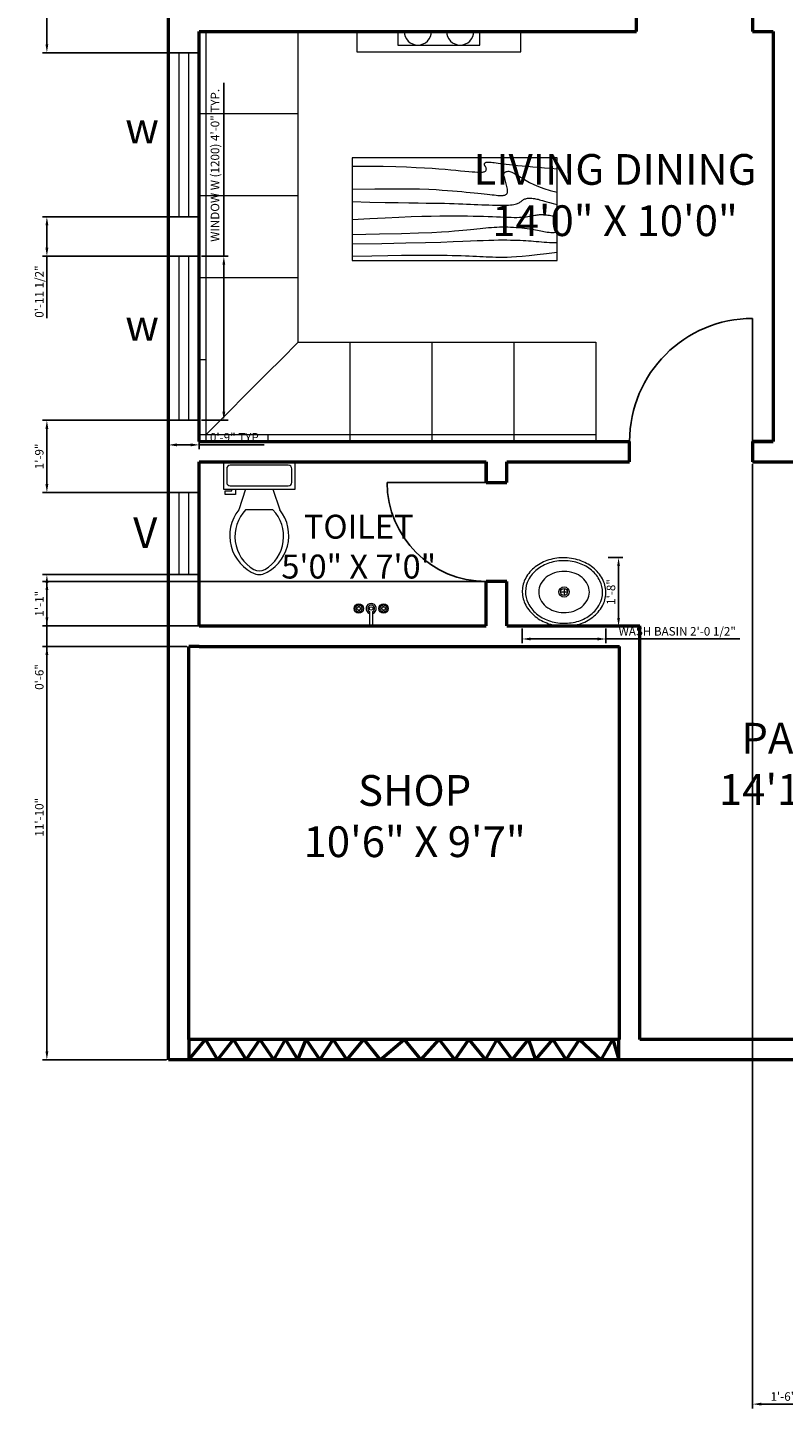
# Model space of a CAD drawing. Units: inches. Extents: x 3688 to 4628, y 1593 to 2337.
# Tile 1 of 7: x 3688 to 3910, y 1593 to 1997. Entities that reach past the tile are written whole.
import ezdxf

# ---------------------------------------------------------------- set-up
doc = ezdxf.new("R2010")
doc.units = ezdxf.units.IN
for name, color, linetype, lineweight in [('A-ANNO-DIMS', 2, 'Continuous', 18), ('A-ANNO-TEXT', 7, 'Continuous', 18), ('A-AREA-IDEN', 7, 'Continuous', 25), ('A-DOOR', 4, 'Continuous', 25), ('A-FLOR-FIXT', 8, 'Continuous', 18), ('A-FURN', 8, 'Continuous', 18), ('A-GLAZ', 4, 'Continuous', 25), ('A-WALL', 7, 'Continuous', 50)]:
    doc.layers.add(name, color=color, linetype=linetype, lineweight=lineweight)
doc.styles.get("Standard").update_dxf_attribs({"font": 'arial.ttf'})
doc.dimstyles.new('ISO-25', dxfattribs={"dimtxt": 2.5, "dimasz": 2.5, "dimexe": 1.25, "dimexo": 0.625, "dimtad": 1, "dimdec": 0, "dimlunit": 3, "dimtxsty": 'Standard', "dimcen": 2.5, "dimadec": 0, "dimazin": 0, "dimtfac": 1, "dimtdec": 0, "dimtmove": 0, "dimatfit": 3, "dimfxl": 1, "dimarcsym": 0})

# ---------------------------------------------------------------- blocks, each defined once
blk = doc.blocks.new('Sink - Oval top')
for p, q in [((-1, 0), (1, 0)), ((0, 1), (0, -1))]:
    blk.add_line(p, q)
for points in [[(-12.23, 0.39, 0.117634), (-11.46, -3.36, 0.104469), (-8.88, -6.8, 0.090016), (-5.08, -9.07, 0.08192), (-0.32, -10.02, 0.08192), (4.49, -9.38, 0.090016), (8.42, -7.36, 0.104469), (11.22, -4.09, 0.117634), (12.23, -0.39, 0.117634), (11.46, 3.36, 0.104469), (8.88, 6.8, 0.090016), (5.08, 9.07, 0.08192), (0.32, 10.02, 0.08192), (-4.49, 9.38, 0.090016), (-8.42, 7.36, 0.104469), (-11.22, 4.09, 0.117634)], [(-11.29, 0.16, 0.118622), (-10.52, -3.25, 0.104678), (-8.07, -6.36, 0.089562), (-4.54, -8.37, 0.081185), (-0.13, -9.15, 0.081185), (4.3, -8.49, 0.089562), (7.89, -6.58, 0.104678), (10.42, -3.55, 0.118622), (11.29, -0.16, 0.118622), (10.52, 3.25, 0.104678), (8.07, 6.36, 0.089562), (4.54, 8.37, 0.081185), (0.13, 9.15, 0.081185), (-4.3, 8.49, 0.089562), (-7.89, 6.58, 0.104678), (-10.42, 3.55, 0.118622)], [(-7.42, 0.08, 0.118283), (-6.91, -2.17, 0.104607), (-5.29, -4.21, 0.089718), (-2.97, -5.53, 0.081436), (-0.07, -6.04, 0.081436), (2.84, -5.59, 0.089718), (5.2, -4.33, 0.104607), (6.86, -2.32, 0.118283), (7.42, -0.08, 0.118283), (6.91, 2.17, 0.104607), (5.29, 4.21, 0.089718), (2.97, 5.53, 0.081436), (0.07, 6.04, 0.081436), (-2.84, 5.59, 0.089718), (-5.2, 4.33, 0.104607), (-6.86, 2.32, 0.118283)]]:
    blk.add_lwpolyline(points, format="xyb", close=True)
for radius in [1.5, 1]:
    blk.add_circle((0, 0), radius)
blk = doc.blocks.new('Toilet - top')
for p, q in [((9.5, -6), (9.5, -2)), ((-8, -8.5), (-8, -8)), ((-7, -8), (-7, -9.5)), ((-4, -8), (-6, -14)), ((4, -8), (6, -14)), ((-10, -8.5), (-8, -8.5)), ((-10, -9.5), (-10, -8.5)), ((-7, -9.5), (-10, -9.5)), ((4, -14), (-4, -14))]:
    blk.add_line(p, q)
blk.add_lwpolyline([(10.5, -8), (10.5, 0), (-10.5, 0), (-10.5, -8)], close=True)
for points in [[(-9.5, -2), (-9.5, -6)], [(8.5, -1), (-8.5, -1)], [(-8.5, -7), (8.5, -7)]]:
    blk.add_lwpolyline(points)
for centre, radius, start, end in [((-8.62, -1.88), 0.884, 81.8699, 188.1301), ((8.62, -1.88), 0.884, 351.8699, 98.1301), ((-8.62, -6.12), 0.884, 171.8699, 278.1301), ((8.62, -6.12), 0.884, 261.8699, 8.1301), ((3.52, -21.58), 12.17, 141.4691, 247.9714), ((4.2, -21.82), 11.33, 136.3677, 238.9468), ((-3.52, -21.58), 12.17, 292.0284, 38.5307), ((-4.2, -21.82), 11.33, 301.053, 43.6321), ((0, -27.88), 4, 245.7318, 294.2682), ((0, -29), 4, 254.8605, 285.1395)]:
    blk.add_arc(centre, radius, start, end)
blk = doc.blocks.new('Table - Rectangular Woodgrain 60 x 30 in.')
for p, q in [((0, 0), (0, -30)), ((60, 0), (0, 0)), ((60, -30), (60, 0)), ((0, -30), (60, -30))]:
    blk.add_line(p, q)
for points in [[(0, -2.4), (4.8155, -2.418), (9.0302, -2.4688), (12.709, -2.5477), (15.9167, -2.65), (18.7181, -2.7711), (21.1781, -2.9063), (23.3616, -3.0508), (25.3333, -3.2), (27.1477, -3.3495), (28.8172, -3.4958), (30.3437, -3.636), (31.7291, -3.7667), (32.9756, -3.8849), (34.0849, -3.9875), (35.059, -4.0714), (35.9, -4.1334), (36.6114, -4.1711), (37.2041, -4.1854), (37.6906, -4.1779), (38.0833, -4.15), (38.3948, -4.1034), (38.6375, -4.0396), (38.8239, -3.9602), (38.9666, -3.8667), (39.0764, -3.7608), (39.1573, -3.6448), (39.2116, -3.521), (39.2416, -3.3917), (39.2498, -3.2593), (39.2385, -3.1261), (39.21, -2.9944), (39.1666, -2.8667), (39.111, -2.7447), (39.0468, -2.6281), (38.978, -2.5163), (38.9083, -2.4083), (38.8418, -2.3035), (38.7823, -2.201), (38.7337, -2.1001), (38.7, -2), (38.6844, -1.9003), (38.6875, -1.8021), (38.7094, -1.707), (38.75, -1.6167), (38.8094, -1.5326), (38.8875, -1.4563), (38.9844, -1.3893), (39.1, -1.3333), (39.2351, -1.2896), (39.3937, -1.2583), (39.5804, -1.2396), (39.8, -1.2333), (40.057, -1.2396), (40.3562, -1.2583), (40.7023, -1.2896), (41.1, -1.3333), (41.5547, -1.3895), (42.0755, -1.4573), (42.6721, -1.5361), (43.3542, -1.625), (44.1316, -1.7233), (45.014, -1.8302), (46.0114, -1.9449), (47.1333, -2.0667), (48.3862, -2.1947), (49.7625, -2.3281), (51.2513, -2.4663), (52.8416, -2.6083), (54.5226, -2.7535), (56.2833, -2.9011), (58.1127, -3.0501), (60, -3.2)], [(0, -9.2), (6.5759, -9.0858), (11.9385, -9.0365), (16.2527, -9.0418), (19.6833, -9.0917), (22.3952, -9.1759), (24.5531, -9.2844), (26.322, -9.4069), (27.8666, -9.5333), (29.3241, -9.6553), (30.7203, -9.7719), (32.0532, -9.8837), (33.3208, -9.9917), (34.5213, -10.0965), (35.6526, -10.199), (36.7128, -10.2999), (37.7, -10.4), (38.6129, -10.4996), (39.4531, -10.5969), (40.223, -10.6895), (40.925, -10.775), (41.5613, -10.8512), (42.1344, -10.9156), (42.6465, -10.966), (43.1, -11), (43.4976, -11.0158), (43.8437, -11.0136), (44.143, -10.9942), (44.4, -10.9583), (44.6195, -10.9069), (44.8062, -10.8406), (44.9648, -10.7603), (45.1, -10.6667), (45.2155, -10.5598), (45.3114, -10.4365), (45.3871, -10.2929), (45.4416, -10.125), (45.4743, -9.929), (45.4844, -9.7011), (45.4709, -9.4371), (45.4333, -9.1333), (45.3716, -8.7883), (45.2896, -8.4104), (45.1919, -8.0107), (45.0833, -7.6), (44.9685, -7.1893), (44.8521, -6.7896), (44.7388, -6.4117), (44.6333, -6.0667), (44.54, -5.7628), (44.4614, -5.4979), (44.4001, -5.2675), (44.3583, -5.0667), (44.3384, -4.8909), (44.3427, -4.7354), (44.3736, -4.5956), (44.4333, -4.4667), (44.5236, -4.3453), (44.6427, -4.2333), (44.7884, -4.1339), (44.9583, -4.05), (45.1501, -3.9849), (45.3614, -3.9417), (45.59, -3.9234), (45.8333, -3.9333), (46.0915, -3.9749), (46.3734, -4.0531), (46.6906, -4.1736), (47.0542, -4.3417), (47.4756, -4.5629), (47.9661, -4.8427), (48.5372, -5.1866), (49.2, -5.6), (49.9676, -6.0844), (50.8594, -6.625), (51.8965, -7.2031), (53.1, -7.8), (54.491, -8.3969), (56.0906, -8.975), (57.9199, -9.5156), (60, -10)], [(0, -12.8), (5.1847, -12.9322), (9.6213, -13.0323), (13.3963, -13.1059), (16.5958, -13.1583), (19.3063, -13.1952), (21.614, -13.2219), (23.6054, -13.2439), (25.3666, -13.2667), (26.9728, -13.2947), (28.4531, -13.3281), (29.8256, -13.3663), (31.1083, -13.4083), (32.3191, -13.4535), (33.476, -13.501), (34.597, -13.5501), (35.7, -13.6), (36.7984, -13.6497), (37.8875, -13.6979), (38.9578, -13.743), (40, -13.7833), (41.0047, -13.8174), (41.9625, -13.8438), (42.864, -13.8607), (43.7, -13.8667), (44.4631, -13.8604), (45.1552, -13.8417), (45.7801, -13.8104), (46.3416, -13.7667), (46.8439, -13.7104), (47.2906, -13.6417), (47.6858, -13.5604), (48.0333, -13.4667), (48.3375, -13.3608), (48.6042, -13.2448), (48.8396, -13.121), (49.05, -12.9917), (49.2417, -12.8593), (49.4208, -12.7261), (49.5937, -12.5944), (49.7667, -12.4667), (49.9452, -12.3451), (50.1323, -12.2313), (50.3303, -12.1268), (50.5416, -12.0333), (50.7686, -11.9524), (51.0135, -11.8854), (51.2788, -11.8341), (51.5666, -11.8), (51.8785, -11.7843), (52.2116, -11.7865), (52.562, -11.8059), (52.926, -11.8417), (53.2998, -11.8931), (53.6795, -11.9594), (54.0614, -12.0397), (54.4416, -12.1333), (54.8223, -12.2401), (55.2293, -12.3625), (55.6942, -12.5037), (56.2489, -12.6667), (56.9251, -12.8547), (57.7545, -13.0708), (58.7689, -13.3182), (60, -13.6)], [(0, -18), (5.124, -17.7273), (9.6609, -17.5057), (13.6705, -17.3303), (17.2125, -17.1958), (20.3467, -17.0973), (23.1328, -17.0297), (25.6307, -16.9878), (27.9, -16.9667), (29.9928, -16.9617), (31.9302, -16.9703), (33.7254, -16.9907), (35.3917, -17.0208), (36.9423, -17.0588), (38.3906, -17.1026), (39.7499, -17.1503), (41.0333, -17.2), (42.2519, -17.2496), (43.4073, -17.2969), (44.4986, -17.3395), (45.525, -17.375), (46.4858, -17.4012), (47.3802, -17.4156), (48.2074, -17.416), (48.9667, -17.4), (49.6583, -17.3662), (50.2872, -17.3167), (50.8595, -17.2547), (51.3812, -17.1833), (51.8584, -17.1057), (52.2971, -17.025), (52.7034, -16.9443), (53.0833, -16.8667), (53.443, -16.7951), (53.789, -16.7313), (54.128, -16.6768), (54.4666, -16.6334), (54.8115, -16.6024), (55.1693, -16.5854), (55.5465, -16.5841), (55.95, -16.6), (56.3828, -16.6337), (56.8346, -16.6823), (57.2915, -16.7418), (57.7396, -16.8084), (58.165, -16.878), (58.5539, -16.9469), (58.8924, -17.0111), (59.1666, -17.0667), (59.3679, -17.1107), (59.5078, -17.1438), (59.6032, -17.1675), (59.6708, -17.1833), (59.7275, -17.193), (59.7901, -17.1979), (59.8753, -17.1998), (60, -17.2)], [(0, -22.4), (8.0098, -22.2501), (14.4094, -22.1011), (19.4168, -21.9535), (23.25, -21.8083), (26.1269, -21.6663), (28.2656, -21.5281), (29.884, -21.3947), (31.2, -21.2667), (32.3967, -21.1448), (33.5172, -21.0292), (34.5697, -20.9198), (35.5625, -20.8167), (36.5037, -20.7198), (37.4015, -20.6292), (38.2642, -20.5448), (39.1, -20.4667), (39.9164, -20.3951), (40.7187, -20.3313), (41.5117, -20.2768), (42.3, -20.2333), (43.0883, -20.2024), (43.8812, -20.1854), (44.6836, -20.1841), (45.5, -20.2), (46.3328, -20.234), (47.1747, -20.2844), (48.0163, -20.3488), (48.8479, -20.425), (49.66, -20.5106), (50.4429, -20.6031), (51.1872, -20.7004), (51.8833, -20.8), (52.5246, -20.8999), (53.1166, -20.9995), (53.6681, -21.0983), (54.1875, -21.1958), (54.6834, -21.2919), (55.1646, -21.3859), (55.6394, -21.4777), (56.1167, -21.5667), (56.6028, -21.6515), (57.0961, -21.7266), (57.5929, -21.7852), (58.0896, -21.8208), (58.5823, -21.8268), (59.0674, -21.7964), (59.5412, -21.723), (60, -21.6)], [(0, -25.2), (8.6355, -25.0504), (15.7026, -24.9031), (21.4049, -24.7606), (25.9458, -24.625), (29.529, -24.4988), (32.3578, -24.3844), (34.6359, -24.284), (36.5667, -24.2), (38.3213, -24.1341), (39.9417, -24.0854), (41.437, -24.0523), (42.8167, -24.0333), (44.0901, -24.0268), (45.2667, -24.0313), (46.3557, -24.0451), (47.3667, -24.0667), (48.309, -24.0947), (49.1928, -24.1287), (50.0284, -24.168), (50.826, -24.2125), (51.5959, -24.2617), (52.3483, -24.3151), (53.0935, -24.3725), (53.8417, -24.4334), (54.6009, -24.497), (55.3699, -24.561), (56.1454, -24.6226), (56.9239, -24.6792), (57.7021, -24.7279), (58.4764, -24.7662), (59.2435, -24.7911), (60, -24.8)], [(0, -28.8), (5.6867, -28.6681), (10.45, -28.5698), (14.407, -28.5012), (17.675, -28.4584), (20.3711, -28.4374), (22.6125, -28.4344), (24.5164, -28.4455), (26.2, -28.4667), (27.762, -28.4947), (29.2276, -28.5281), (30.6033, -28.5663), (31.8958, -28.6084), (33.1118, -28.6535), (34.2578, -28.7011), (35.3405, -28.7501), (36.3666, -28.8), (37.3443, -28.8497), (38.288, -28.8974), (39.2137, -28.9412), (40.1375, -28.9792), (41.0753, -29.0093), (42.0432, -29.0297), (43.0572, -29.0384), (44.1333, -29.0333), (45.2936, -29.0114), (46.5843, -28.9641), (48.0579, -28.8816), (49.7666, -28.7542), (51.7629, -28.5721), (54.0989, -28.3255), (56.8272, -28.0048), (60, -27.6)]]:
    blk.add_lwpolyline(points)
blk = doc.blocks.new('Faucet - Bathroom top')
for p, q in [((-4.107, 0.125), (-4.375, 0.125)), ((-3.75, 0.4788), (-3.75, 0.75)), ((-3.5, 0.482), (-3.5, 0.75)), ((-3.1461, 0.125), (-2.875, 0.125)), ((3.143, 0.125), (2.875, 0.125)), ((3.5, 0.4788), (3.5, 0.75)), ((3.75, 0.482), (3.75, 0.75)), ((4.1039, 0.125), (4.375, 0.125)), ((-4.1039, -0.125), (-4.375, -0.125)), ((-3.75, -0.4821), (-3.75, -0.75)), ((-3.5, -0.4789), (-3.5, -0.75)), ((-3.143, -0.125), (-2.875, -0.125)), ((-0.5, -0.8639), (-0.5, -4.5)), ((0.5, -4.5), (0.5, -0.8631)), ((3.1461, -0.125), (2.875, -0.125)), ((3.5, -0.4821), (3.5, -0.75)), ((3.75, -0.4789), (3.75, -0.75)), ((4.107, -0.125), (4.375, -0.125))]:
    blk.add_line(p, q)
for centre, radius in [((-3.625, 0), 1.375), ((-4.625, 0), 0.2795), ((-3.625, 0), 0.5), ((-3.625, 1), 0.2795), ((-2.625, 0), 0.2795), ((0, 0), 0.5), ((3.625, 0), 1.375), ((2.625, 0), 0.2795), ((3.625, 0), 0.5), ((3.625, 1), 0.2795), ((4.625, 0), 0.2795), ((-3.625, -1), 0.2795), ((3.625, -1), 0.2795)]:
    blk.add_circle(centre, radius)
for centre, radius, start, end in [((-3.625, 0), 1, 105.2407, 164.2093), ((-3.625, 0), 1, 16.44125, 74.07887), ((0, 0), 1.5, 289.6514, 250.3603), ((0, 0), 1, 300.3431, 239.7554), ((3.625, 0), 1, 106.12, 164.0884), ((3.625, 0), 1, 16.23422, 73.90469), ((-3.625, 0), 1, 196.2342, 253.9047), ((-3.625, 0), 1, 286.12, 344.0884), ((3.625, 0), 1, 196.4413, 254.0789), ((3.625, 0), 1, 285.2407, 344.2093), ((0, -4.5), 0.5, 180, 0)]:
    blk.add_arc(centre, radius, start, end)
blk = doc.blocks.new('DOOR-900')
blk.add_line((0, 0), (0, 36))
blk.add_arc((0, 0), 36, 0, 90)
blk = doc.blocks.new('DOOR-750')
blk.add_line((29, 0), (29, 29))
blk.add_arc((29, 0), 29, 90, 180)
blk = doc.blocks.new('WIN-1200')
for p, q in [((0, 48), (0, 0)), ((9, 48), (0, 48)), ((9, 0), (9, 48)), ((0, 0), (9, 0))]:
    blk.add_line(p, q)
blk = doc.blocks.new('WIN-600')
for p, q in [((24, 9), (0, 9)), ((0, 9), (0, 0)), ((24, 0), (24, 9)), ((0, 0), (24, 0))]:
    blk.add_line(p, q)
blk = doc.blocks.new('*D23')
at = {"layer": 'A-ANNO-DIMS', "color": 0, "lineweight": -2, "transparency": 16777216}
for p, q in [((3745.82, 1930.49), (3745.82, 1981.21)), ((3739.25, 1930.49), (3747.07, 1930.49)), ((3745.82, 1884.99), (3745.82, 1927.99)), ((3739.25, 1882.49), (3747.07, 1882.49))]:
    blk.add_line(p, q, dxfattribs=at)
at = {"layer": 'A-ANNO-DIMS', "color": 0, "transparency": 16777216}
for points in [[(3745.41, 1927.99), (3746.24, 1927.99), (3745.82, 1930.49)], [(3745.41, 1884.99), (3746.24, 1884.99), (3745.82, 1882.49)]]:
    blk.add_solid(points, dxfattribs=at)
at = {"layer": 'Defpoints', "color": 0, "transparency": 16777216}
for p in [(3738.62, 1930.49), (3745.82, 1930.49), (3738.62, 1882.49)]:
    blk.add_point(p, dxfattribs=at)
at = {"layer": 'A-ANNO-DIMS', "color": 0, "transparency": 16777216, "insert": (3743.56, 1957.1), "char_height": 2.5, "attachment_point": 5, "rotation": 90}
blk.add_mtext('WINDOW W (1200) 4\'-0" TYP.', dxfattribs=at)
blk = doc.blocks.new('*D24')
at = {"layer": 'A-ANNO-DIMS', "color": 0, "lineweight": -2, "transparency": 16777216}
for p, q in [((3729.62, 1881.87), (3729.62, 1874.04)), ((3738.62, 1881.87), (3738.62, 1874.04)), ((3732.12, 1875.29), (3736.12, 1875.29)), ((3738.62, 1875.29), (3757.61, 1875.29))]:
    blk.add_line(p, q, dxfattribs=at)
at = {"layer": 'A-ANNO-DIMS', "color": 0, "transparency": 16777216}
for points in [[(3732.12, 1875.71), (3732.12, 1874.87), (3729.62, 1875.29)], [(3736.12, 1875.71), (3736.12, 1874.87), (3738.62, 1875.29)]]:
    blk.add_solid(points, dxfattribs=at)
at = {"layer": 'Defpoints', "color": 0, "transparency": 16777216}
for p in [(3729.62, 1882.49), (3738.62, 1882.49), (3738.62, 1875.29)]:
    blk.add_point(p, dxfattribs=at)
at = {"layer": 'A-ANNO-DIMS', "color": 0, "transparency": 16777216, "insert": (3749.37, 1877.19), "char_height": 2.5, "attachment_point": 5}
blk.add_mtext('0\'-9" TYP.', dxfattribs=at)
blk = doc.blocks.new('*D47')
at = {"layer": 'A-ANNO-DIMS', "color": 0, "lineweight": -2, "transparency": 16777216}
for p, q in [((3833.14, 1821.55), (3833.14, 1817.24)), ((3835.64, 1818.49), (3855.19, 1818.49)), ((3857.69, 1821.55), (3857.69, 1817.24)), ((3857.69, 1818.49), (3896.91, 1818.49))]:
    blk.add_line(p, q, dxfattribs=at)
at = {"layer": 'A-ANNO-DIMS', "color": 0, "transparency": 16777216}
for points in [[(3835.64, 1818.91), (3835.64, 1818.07), (3833.14, 1818.49)], [(3855.19, 1818.91), (3855.19, 1818.07), (3857.69, 1818.49)]]:
    blk.add_solid(points, dxfattribs=at)
at = {"layer": 'Defpoints', "color": 0, "transparency": 16777216}
for p in [(3833.14, 1822.17), (3857.69, 1822.17), (3857.69, 1818.49)]:
    blk.add_point(p, dxfattribs=at)
at = {"layer": 'A-ANNO-DIMS', "color": 0, "transparency": 16777216, "insert": (3878.55, 1820.41), "char_height": 2.5, "attachment_point": 5}
blk.add_mtext('WASH BASIN 2\'-0 1/2"', dxfattribs=at)
blk = doc.blocks.new('*D48')
at = {"layer": 'A-ANNO-DIMS', "color": 0, "lineweight": -2, "transparency": 16777216}
for p, q in [((3858.31, 1842.31), (3862.62, 1842.31)), ((3861.37, 1824.67), (3861.37, 1839.81)), ((3858.31, 1822.17), (3862.62, 1822.17))]:
    blk.add_line(p, q, dxfattribs=at)
at = {"layer": 'A-ANNO-DIMS', "color": 0, "transparency": 16777216}
for points in [[(3860.96, 1839.81), (3861.79, 1839.81), (3861.37, 1842.31)], [(3860.96, 1824.67), (3861.79, 1824.67), (3861.37, 1822.17)]]:
    blk.add_solid(points, dxfattribs=at)
at = {"layer": 'Defpoints', "color": 0, "transparency": 16777216}
for p in [(3857.69, 1842.31), (3861.37, 1842.31), (3857.69, 1822.17)]:
    blk.add_point(p, dxfattribs=at)
at = {"layer": 'A-ANNO-DIMS', "color": 0, "transparency": 16777216, "insert": (3859.47, 1832.24), "char_height": 2.5, "attachment_point": 5, "rotation": 90}
blk.add_mtext('1\'-8"', dxfattribs=at)
blk = doc.blocks.new('*D53')
at = {"layer": 'A-ANNO-DIMS', "color": 0, "lineweight": -2, "transparency": 16777216}
for p, q in [((3729, 2029.26), (3692.77, 2029.26)), ((3694.02, 2026.76), (3694.02, 1992.54)), ((3729, 1990.04), (3692.77, 1990.04))]:
    blk.add_line(p, q, dxfattribs=at)
at = {"layer": 'A-ANNO-DIMS', "color": 0, "transparency": 16777216}
for points in [[(3693.61, 2026.76), (3694.44, 2026.76), (3694.02, 2029.26)], [(3693.61, 1992.54), (3694.44, 1992.54), (3694.02, 1990.04)]]:
    blk.add_solid(points, dxfattribs=at)
at = {"layer": 'Defpoints', "color": 0, "transparency": 16777216}
for p in [(3729.62, 2029.26), (3694.02, 1990.04), (3729.62, 1990.04)]:
    blk.add_point(p, dxfattribs=at)
at = {"layer": 'A-ANNO-DIMS', "color": 0, "transparency": 16777216, "insert": (3692.12, 2009.65), "char_height": 2.5, "attachment_point": 5, "rotation": 90}
blk.add_mtext('3\'-3"', dxfattribs=at)
blk = doc.blocks.new('*D54')
at = {"layer": 'A-ANNO-DIMS', "color": 0, "lineweight": -2, "transparency": 16777216}
for p, q in [((3729, 1942.04), (3692.77, 1942.04)), ((3694.02, 1939.54), (3694.02, 1932.99)), ((3729, 1930.49), (3692.77, 1930.49)), ((3694.02, 1930.49), (3694.02, 1912.33))]:
    blk.add_line(p, q, dxfattribs=at)
at = {"layer": 'A-ANNO-DIMS', "color": 0, "transparency": 16777216}
for points in [[(3693.61, 1939.54), (3694.44, 1939.54), (3694.02, 1942.04)], [(3693.61, 1932.99), (3694.44, 1932.99), (3694.02, 1930.49)]]:
    blk.add_solid(points, dxfattribs=at)
at = {"layer": 'Defpoints', "color": 0, "transparency": 16777216}
for p in [(3729.62, 1942.04), (3694.02, 1930.49), (3729.62, 1930.49)]:
    blk.add_point(p, dxfattribs=at)
at = {"layer": 'A-ANNO-DIMS', "color": 0, "transparency": 16777216, "insert": (3692.11, 1920.16), "char_height": 2.5, "attachment_point": 5, "rotation": 90}
blk.add_mtext('0\'-11 1/2"', dxfattribs=at)
blk = doc.blocks.new('*D55')
at = {"layer": 'A-ANNO-DIMS', "color": 0, "lineweight": -2, "transparency": 16777216}
for p, q in [((3729, 1882.49), (3692.77, 1882.49)), ((3694.02, 1879.99), (3694.02, 1863.83)), ((3729, 1861.33), (3692.77, 1861.33))]:
    blk.add_line(p, q, dxfattribs=at)
at = {"layer": 'A-ANNO-DIMS', "color": 0, "transparency": 16777216}
for points in [[(3693.61, 1879.99), (3694.44, 1879.99), (3694.02, 1882.49)], [(3693.61, 1863.83), (3694.44, 1863.83), (3694.02, 1861.33)]]:
    blk.add_solid(points, dxfattribs=at)
at = {"layer": 'Defpoints', "color": 0, "transparency": 16777216}
for p in [(3729.62, 1882.49), (3694.02, 1861.33), (3729.62, 1861.33)]:
    blk.add_point(p, dxfattribs=at)
at = {"layer": 'A-ANNO-DIMS', "color": 0, "transparency": 16777216, "insert": (3692.12, 1871.91), "char_height": 2.5, "attachment_point": 5, "rotation": 90}
blk.add_mtext('1\'-9"', dxfattribs=at)
blk = doc.blocks.new('*D56')
at = {"layer": 'A-ANNO-DIMS', "color": 0, "lineweight": -2, "transparency": 16777216}
for p, q in [((3729, 1837.33), (3692.77, 1837.33)), ((3694.02, 1834.83), (3694.02, 1697.82)), ((3729, 1695.32), (3692.77, 1695.32))]:
    blk.add_line(p, q, dxfattribs=at)
at = {"layer": 'A-ANNO-DIMS', "color": 0, "transparency": 16777216}
for points in [[(3693.61, 1834.83), (3694.44, 1834.83), (3694.02, 1837.33)], [(3693.61, 1697.82), (3694.44, 1697.82), (3694.02, 1695.32)]]:
    blk.add_solid(points, dxfattribs=at)
at = {"layer": 'Defpoints', "color": 0, "transparency": 16777216}
for p in [(3729.62, 1837.33), (3694.02, 1695.32), (3729.62, 1695.32)]:
    blk.add_point(p, dxfattribs=at)
at = {"layer": 'A-ANNO-DIMS', "color": 0, "transparency": 16777216, "insert": (3692.12, 1766.32), "char_height": 2.5, "attachment_point": 5, "rotation": 90}
blk.add_mtext('11\'-10"', dxfattribs=at)
blk = doc.blocks.new('*D72')
at = {"layer": 'A-ANNO-DIMS', "color": 0, "lineweight": -2, "transparency": 16777216}
for p, q in [((3900.62, 1869.69), (3900.62, 1593.32)), ((3918.62, 1869.69), (3918.62, 1593.32)), ((3903.12, 1594.57), (3916.12, 1594.57))]:
    blk.add_line(p, q, dxfattribs=at)
at = {"layer": 'A-ANNO-DIMS', "color": 0, "transparency": 16777216}
for points in [[(3903.12, 1594.98), (3903.12, 1594.15), (3900.62, 1594.57)], [(3916.12, 1594.98), (3916.12, 1594.15), (3918.62, 1594.57)]]:
    blk.add_solid(points, dxfattribs=at)
at = {"layer": 'Defpoints', "color": 0, "transparency": 16777216}
for p in [(3900.62, 1870.32), (3918.62, 1870.32), (3918.62, 1594.57)]:
    blk.add_point(p, dxfattribs=at)
at = {"layer": 'A-ANNO-DIMS', "color": 0, "transparency": 16777216, "insert": (3909.62, 1596.47), "char_height": 2.5, "attachment_point": 5}
blk.add_mtext('1\'-6"', dxfattribs=at)
blk = doc.blocks.new('*D73')
at = {"layer": 'A-ANNO-DIMS', "color": 0, "lineweight": -2, "transparency": 16777216}
for p, q in [((3694.02, 1824.82), (3694.02, 1827.32)), ((3738, 1822.32), (3692.77, 1822.32)), ((3694.02, 1822.32), (3694.02, 1816.32)), ((3735, 1816.32), (3692.77, 1816.32)), ((3694.02, 1813.82), (3694.02, 1803.42))]:
    blk.add_line(p, q, dxfattribs=at)
at = {"layer": 'A-ANNO-DIMS', "color": 0, "transparency": 16777216}
for points in [[(3693.61, 1824.82), (3694.44, 1824.82), (3694.02, 1822.32)], [(3693.61, 1813.82), (3694.44, 1813.82), (3694.02, 1816.32)]]:
    blk.add_solid(points, dxfattribs=at)
at = {"layer": 'Defpoints', "color": 0, "transparency": 16777216}
for p in [(3738.62, 1822.32), (3694.02, 1816.32), (3735.62, 1816.32)]:
    blk.add_point(p, dxfattribs=at)
at = {"layer": 'A-ANNO-DIMS', "color": 0, "transparency": 16777216, "insert": (3692.12, 1807.37), "char_height": 2.5, "attachment_point": 5, "rotation": 90}
blk.add_mtext('0\'-6"', dxfattribs=at)
blk = doc.blocks.new('*D74')
at = {"layer": 'A-ANNO-DIMS', "color": 0, "lineweight": -2, "transparency": 16777216}
for p, q in [((3822, 1835.32), (3692.77, 1835.32)), ((3694.02, 1832.82), (3694.02, 1824.82)), ((3822, 1822.32), (3692.77, 1822.32))]:
    blk.add_line(p, q, dxfattribs=at)
at = {"layer": 'A-ANNO-DIMS', "color": 0, "transparency": 16777216}
for points in [[(3693.61, 1832.82), (3694.44, 1832.82), (3694.02, 1835.32)], [(3693.61, 1824.82), (3694.44, 1824.82), (3694.02, 1822.32)]]:
    blk.add_solid(points, dxfattribs=at)
at = {"layer": 'Defpoints', "color": 0, "transparency": 16777216}
for p in [(3822.62, 1835.32), (3694.02, 1822.32), (3822.62, 1822.32)]:
    blk.add_point(p, dxfattribs=at)
at = {"layer": 'A-ANNO-DIMS', "color": 0, "transparency": 16777216, "insert": (3692.14, 1828.82), "char_height": 2.5, "attachment_point": 5, "rotation": 90}
blk.add_mtext('1\'-1"', dxfattribs=at)

msp = doc.modelspace()

# ---------------------------------------------------------------- linework, layer by layer
at = {"layer": 'A-FURN'}
for p, q in [((3740.62, 1876.32), (3740.62, 1996.32)), ((3767.62, 1905.32), (3767.62, 1996.32)), ((3784.77, 1996.32), (3784.77, 1993.32)), ((3784.77, 1996.32), (3796.77, 1996.32)), ((3796.77, 1996.32), (3796.77, 1992.32)), ((3820.77, 1992.32), (3820.77, 1996.32)), ((3832.77, 1990.32), (3832.77, 1996.32)), ((3784.77, 1993.32), (3784.77, 1990.32)), ((3796.77, 1992.32), (3820.77, 1992.32)), ((3732.62, 1990.04), (3732.62, 1942.04)), ((3735.62, 1942.04), (3735.62, 1990.04)), ((3784.77, 1990.32), (3832.77, 1990.32)), ((3738.62, 1972.32), (3767.62, 1972.32)), ((3738.62, 1948.32), (3767.62, 1948.32)), ((3732.62, 1930.49), (3732.62, 1882.49)), ((3735.62, 1882.49), (3735.62, 1930.49)), ((3738.62, 1924.32), (3767.62, 1924.32)), ((3767.62, 1905.32), (3762.62, 1900.32)), ((3767.62, 1905.32), (3854.73, 1905.32)), ((3782.73, 1905.32), (3782.73, 1876.32)), ((3806.73, 1905.32), (3806.73, 1876.32)), ((3830.73, 1905.32), (3830.73, 1876.32)), ((3854.73, 1905.32), (3854.73, 1876.32)), ((3738.62, 1900.32), (3740.62, 1900.32)), ((3758.73, 1896.43), (3762.62, 1900.32)), ((3758.73, 1896.43), (3740.62, 1878.32)), ((3738.62, 1878.32), (3854.73, 1878.32)), ((3758.73, 1878.32), (3758.73, 1876.32)), ((3732.62, 1861.33), (3732.62, 1837.33)), ((3735.62, 1837.33), (3735.62, 1861.33))]:
    msp.add_line(p, q, dxfattribs=at)
for centre in [(3802.62, 1996.32), (3815.02, 1996.32)]:
    msp.add_arc(centre, 4, 180, 0, dxfattribs=at)
at = {"layer": 'A-WALL'}
for p, q in [((3729.62, 1695.32), (3729.62, 2295.32)), ((3866.62, 1996.32), (3866.62, 2002.32)), ((3900.62, 2002.32), (3900.62, 1996.32)), ((3738.62, 1996.32), (3866.62, 1996.32)), ((3738.62, 1876.32), (3738.62, 1996.32)), ((3900.62, 1996.32), (3906.62, 1996.32)), ((3906.62, 1996.32), (3906.62, 1876.32)), ((3738.62, 1876.32), (3864.62, 1876.32)), ((3864.62, 1870.32), (3864.62, 1876.32)), ((3906.62, 1876.32), (3900.62, 1876.32)), ((3900.62, 1876.32), (3900.62, 1870.32)), ((3900.62, 1876.32), (3906.62, 1876.32)), ((3738.62, 1870.32), (3798.62, 1870.32)), ((3738.62, 1822.32), (3738.62, 1870.32)), ((3798.62, 1870.32), (3804.62, 1870.32)), ((3804.62, 1870.32), (3822.62, 1870.32)), ((3822.62, 1870.32), (3822.62, 1864.32)), ((3822.62, 1864.32), (3822.62, 1870.32)), ((3828.62, 1870.32), (3864.62, 1870.32)), ((3828.62, 1864.32), (3828.62, 1870.32)), ((3900.62, 1870.32), (3918.62, 1870.32)), ((3822.62, 1864.32), (3828.62, 1864.32)), ((3822.62, 1822.32), (3822.62, 1835.32)), ((3828.62, 1835.32), (3822.62, 1835.32)), ((3828.62, 1822.32), (3828.62, 1835.32)), ((3738.62, 1822.32), (3798.62, 1822.32)), ((3798.62, 1822.32), (3804.62, 1822.32)), ((3804.62, 1822.32), (3822.62, 1822.32)), ((3828.62, 1822.32), (3861.62, 1822.32)), ((3861.62, 1822.32), (3867.62, 1822.32)), ((3867.62, 1701.32), (3867.62, 1822.32)), ((3738.62, 1816.32), (3735.62, 1816.32)), ((3735.62, 1701.32), (3735.62, 1816.32)), ((3738.62, 1816.32), (3804.62, 1816.32)), ((3804.62, 1816.32), (3861.62, 1816.32)), ((3861.62, 1701.32), (3861.62, 1816.32)), ((3861.62, 1701.32), (3735.62, 1701.32)), ((3735.62, 1701.32), (3735.62, 1695.32)), ((3735.62, 1695.32), (3740.43, 1701.32)), ((3861.44, 1701.32), (3735.62, 1701.32)), ((3740.43, 1701.32), (3743.97, 1695.32)), ((3743.97, 1695.32), (3748.62, 1701.32)), ((3748.62, 1701.32), (3752.35, 1695.32)), ((3752.35, 1695.32), (3756.34, 1701.32)), ((3756.34, 1701.32), (3760.5, 1695.32)), ((3760.5, 1695.32), (3763.92, 1701.32)), ((3763.92, 1701.32), (3767.53, 1695.32)), ((3767.53, 1695.32), (3769.95, 1701.32)), ((3769.95, 1701.32), (3773.91, 1695.32)), ((3773.91, 1695.32), (3777.79, 1701.32)), ((3777.79, 1701.32), (3781.86, 1695.32)), ((3781.86, 1695.32), (3786.81, 1701.32)), ((3786.81, 1701.32), (3791.63, 1695.32)), ((3791.63, 1695.32), (3798.62, 1701.32)), ((3798.62, 1701.32), (3803.52, 1695.32)), ((3803.52, 1695.32), (3808.83, 1701.32)), ((3808.83, 1701.32), (3813.46, 1695.32)), ((3813.46, 1695.32), (3817.58, 1701.32)), ((3817.58, 1701.32), (3822.4, 1695.32)), ((3822.4, 1695.32), (3825.84, 1701.32)), ((3825.84, 1701.32), (3830.27, 1695.32)), ((3830.27, 1695.32), (3834.99, 1701.32)), ((3834.99, 1701.32), (3837.05, 1695.32)), ((3837.05, 1695.32), (3842.16, 1701.32)), ((3842.16, 1701.32), (3846, 1695.32)), ((3846, 1695.32), (3849.93, 1701.32)), ((3849.93, 1701.32), (3856.32, 1695.32)), ((3856.32, 1695.32), (3859.67, 1701.32)), ((3859.67, 1701.32), (3861.44, 1695.32)), ((3861.44, 1695.32), (3861.44, 1701.32)), ((4089.62, 1701.32), (3867.62, 1701.32)), ((4089.62, 1695.32), (3729.62, 1695.32))]:
    msp.add_line(p, q, dxfattribs=at)

# ---------------------------------------------------------------- block references
at = {"layer": 'A-DOOR', "extrusion": (0, 0, -1), "zscale": -1}
msp.add_blockref('DOOR-900', (-3900.62, 1876.32), dxfattribs=at)
at = {"layer": 'A-DOOR', "rotation": 89.99999999999685}
msp.add_blockref('DOOR-750', (3822.62, 1835.32), dxfattribs=at)
at = {"layer": 'A-FLOR-FIXT'}
for name, p in [('Toilet - top', (3756.2, 1870.32)), ('Sink - Oval top', (3845.41, 1832.24)), ('Faucet - Bathroom top', (3788.95, 1827.4))]:
    msp.add_blockref(name, p, dxfattribs=at)
at = {"layer": 'A-FURN'}
msp.add_blockref('Table - Rectangular Woodgrain 60 x 30 in.', (3783.42, 1959.29), dxfattribs=at)
at = {"layer": 'A-GLAZ'}
for p in [(3729.62, 1942.04), (3729.62, 1882.49)]:
    msp.add_blockref('WIN-1200', p, dxfattribs=at)
at = {"layer": 'A-GLAZ', "rotation": 270}
msp.add_blockref('WIN-600', (3729.62, 1861.33), dxfattribs=at)

# ---------------------------------------------------------------- texts
at = {"layer": 'A-ANNO-TEXT', "char_height": 9, "attachment_point": 1}
for s, heights, insert in [('\\pxqc;w', [0], (3652.65, 1972.57)), ('\\pxqc;w', [0], (3652.66, 1914.83)), ('\\pxqc;V', [37.18], (3653.57, 1854.07))]:
    msp.add_mtext_dynamic_manual_height_columns(s, width=138.4723, gutter_width=12.5, heights=heights, dxfattribs=dict(at, insert=insert))
at = {"layer": 'A-AREA-IDEN', "attachment_point": 1}
for s, width, insert, char_height in [('\\pxqc;LIVING DINING\\P14\'0" X 10\'0"', 105.0766, (3807.81, 1960.41), 9), ('\\pxqc;TOILET \\P5\'0" X 7\'0"', 61.3205, (3754.65, 1854.85), 7), ('\\pxqc;PARKING \\P14\'1" X 8\'9" ', 105.0766, (3870.74, 1793.95), 9), ('\\pxqc;SHOP^J10\'6" X 9\'7"', 105.0766, (3749.14, 1778.66), 9)]:
    msp.add_mtext_dynamic_manual_height_columns(s, width=width, gutter_width=12.5, heights=[0], dxfattribs=dict(at, insert=insert, char_height=char_height))

# ---------------------------------------------------------------- dimensions: what is measured, and where the dimension line sits
at = {"layer": 'A-ANNO-DIMS'}
for base, p1, p2, override, picture, middle in [((3694.02, 1990.04), (3729.62, 2029.26), (3729.62, 1990.04), {"dimdec": 1, "dimlfac": 1, "dimrnd": 0, "dimzin": 1, "dimdsep": 46, "dimlunit": 4, "dimfrac": 2}, '*D53', (3692.12, 2009.65)), ((3694.0237, 1930.4912), (3729.6237, 1942.0408), (3729.6237, 1930.4912), {"dimdec": 1, "dimlfac": 1, "dimrnd": 0, "dimzin": 1, "dimdsep": 46, "dimlunit": 4, "dimfrac": 2}, '*D54', (3692.106, 1920.1595)), ((3694.02, 1861.33), (3729.62, 1882.49), (3729.62, 1861.33), {"dimdec": 1, "dimlfac": 1, "dimrnd": 0, "dimzin": 1, "dimdsep": 46, "dimlunit": 4, "dimfrac": 2}, '*D55', (3692.12, 1871.91)), ((3861.37, 1842.31), (3857.69, 1822.17), (3857.69, 1842.31), {"dimdec": 1, "dimrnd": 0, "dimzin": 1, "dimlunit": 4, "dimfrac": 2}, '*D48', (3859.47, 1832.24)), ((3694.02, 1695.32), (3729.62, 1837.33), (3729.62, 1695.32), {"dimdec": 1, "dimlfac": 1, "dimrnd": 0, "dimzin": 1, "dimdsep": 46, "dimlunit": 4, "dimfrac": 2}, '*D56', (3692.12, 1766.32)), ((3694.02, 1822.32), (3822.62, 1835.32), (3822.62, 1822.32), {"dimdec": 1, "dimlfac": 1, "dimrnd": 0, "dimzin": 1, "dimdsep": 46, "dimlunit": 4, "dimfrac": 2}, '*D74', (3692.14, 1828.82)), ((3694.02, 1816.32), (3738.62, 1822.32), (3735.62, 1816.32), {"dimdec": 1, "dimlfac": 1, "dimrnd": 0, "dimzin": 1, "dimdsep": 46, "dimlunit": 4, "dimfrac": 2}, '*D73', (3692.12, 1807.37))]:
    dim = msp.add_linear_dim(base=base, p1=p1, p2=p2, angle=90, dimstyle='ISO-25', override=override, dxfattribs=at)
    dim.commit()
    dim.dimension.update_dxf_attribs({"geometry": picture, "text_midpoint": middle})
dim = msp.add_linear_dim(base=(3745.82, 1930.49), p1=(3738.62, 1882.49), p2=(3738.62, 1930.49), angle=90, text='WINDOW W (1200) <> TYP.', dimstyle='ISO-25', override={"dimdec": 1, "dimrnd": 0, "dimzin": 1, "dimlunit": 4, "dimfrac": 2}, dxfattribs=at)
dim.commit()
dim.dimension.update_dxf_attribs({"geometry": '*D23', "text_midpoint": (3743.56, 1957.1)})
for base, p1, p2, text, picture, middle in [((3738.62, 1875.29), (3729.62, 1882.49), (3738.62, 1882.49), '<> TYP.', '*D24', (3749.37, 1877.19)), ((3857.6895, 1818.4894), (3833.1386, 1822.172), (3857.6895, 1822.172), 'WASH BASIN <>', '*D47', (3878.5507, 1820.407))]:
    dim = msp.add_linear_dim(base=base, p1=p1, p2=p2, text=text, dimstyle='ISO-25', override={"dimdec": 1, "dimrnd": 0, "dimzin": 1, "dimlunit": 4, "dimfrac": 2}, dxfattribs=at)
    dim.commit()
    dim.dimension.update_dxf_attribs({"geometry": picture, "text_midpoint": middle})
dim = msp.add_linear_dim(base=(3918.62, 1594.57), p1=(3900.62, 1870.32), p2=(3918.62, 1870.32), dimstyle='ISO-25', override={"dimdec": 1, "dimlfac": 1, "dimrnd": 0, "dimzin": 1, "dimdsep": 46, "dimlunit": 4, "dimfrac": 2}, dxfattribs=at)
dim.commit()
dim.dimension.update_dxf_attribs({"geometry": '*D72', "text_midpoint": (3909.62, 1596.47)})

doc.saveas('drawing.dxf')
